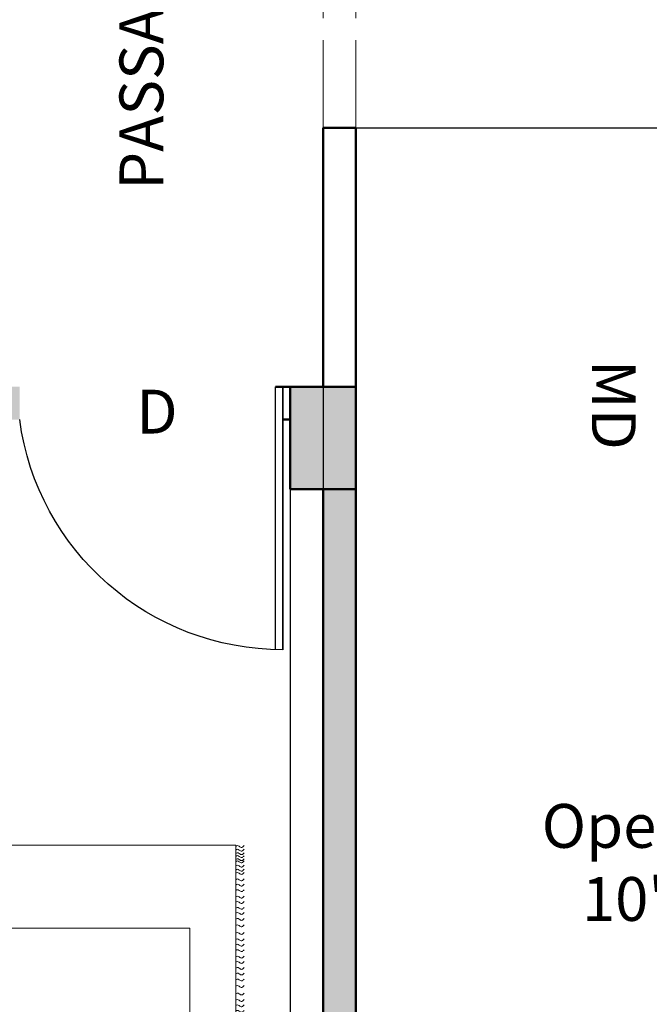
# Model space of a CAD drawing. Units: inches. Extents: x 1601 to 2080, y 5000 to 5589.
# Tile 4 of 11: x 1788 to 1874, y 5125 to 5259. Entities that reach past the tile are written whole.
import ezdxf

# ---------------------------------------------------------------- set-up
doc = ezdxf.new("R2010")
doc.units = ezdxf.units.IN
doc.header["$MEASUREMENT"] = 0
doc.linetypes.add('ACAD_ISO02W100', pattern=[15, 12, -3])
for name, color, linetype, lineweight in [('A-ANNO-DIMS', 2, 'Continuous', 18), ('A-ANNO-TEXT', 7, 'Continuous', 25), ('A-AREA-IDEN', 7, 'Continuous', 25), ('A-COLS', 7, 'Continuous', 50), ('A-COLS-PATT', 18, 'Continuous', 13), ('A-DOOR', 3, 'Continuous', 25), ('A-FLOR-PATT', 8, 'Continuous', 13), ('A-FURN', 8, 'Continuous', 18), ('A-WALL', 7, 'Continuous', 50), ('A-WALL-OVHD', 7, 'ACAD_ISO02W100', 18), ('A-WALL-PATT', 241, 'Continuous', 13)]:
    doc.layers.add(name, color=color, linetype=linetype, lineweight=lineweight)
doc.styles.get("Standard").update_dxf_attribs({"font": 'arial.ttf'})
doc.dimstyles.get("Standard").update_dxf_attribs({"dimtxt": 6, "dimasz": 0.18, "dimexe": 0.18, "dimexo": 0.0625, "dimgap": 0.09, "dimtad": 0, "dimtih": 1, "dimtoh": 1, "dimdec": 1, "dimzin": 0, "dimdsep": 46, "dimlunit": 3, "dimtxsty": 'Standard', "dimcen": 0.09, "dimadec": 0, "dimazin": 0, "dimtfac": 1, "dimtdec": 1, "dimtofl": 0, "dimtmove": 0, "dimatfit": 3, "dimfxl": 1, "dimtolj": 1, "dimtzin": 0, "dimarcsym": 0})

# ---------------------------------------------------------------- blocks, each defined once
blk = doc.blocks.new('BED-DOUBLE-ENSEMBLE')
for p, q in [((5.6, 61.61), (5.6, 51.56)), ((63.65, 61.72), (63.65, 51.66)), ((68.68, 56.69), (58.62, 56.69)), ((10.63, 56.59), (0.57, 56.59)), ((49.39, 52.82), (10.63, 52.82)), ((49.39, 52.82), (58, 46.47)), ((49.44, 52.82), (49.44, 46.47)), ((49.44, 52), (10.63, 52)), ((49.44, 46.47), (58, 46.47)), ((58.05, 34.96), (10.63, 34.96)), ((4.35, 0), (4.35, 26.37)), ((4.35, 26.37), (10.65, 26.37)), ((58.05, 26.37), (67.59, 26.37)), ((67.59, 26.37), (67.59, 0)), ((67.59, 0), (4.35, 0))]:
    blk.add_line(p, q)
for points in [[(0, 50.39), (10.63, 50.5), (10.63, 62.68), (0, 62.58)], [(58.05, 62.68), (58.05, 11.36), (10.63, 11.36), (10.63, 62.68)], [(58.05, 50.5), (68.68, 50.6), (68.68, 62.78), (58.05, 62.68)], [(29.88, 59.98), (29.88, 52.82), (15.98, 52.82), (15.98, 59.98)], [(49.44, 59.98), (49.44, 52.82), (35.55, 52.82), (35.55, 59.98)]]:
    blk.add_lwpolyline(points, close=True)
for centre in [(5.6, 56.59), (63.65, 56.69)]:
    blk.add_circle(centre, 3.92)
for points, knots in [([(3.23, 25.83), (3.32, 25.96), (3.52, 26.2), (3.86, 25.96), (4.14, 25.78), (4.29, 25.89), (4.35, 25.94)], [0, 0, 0, 0, 0.400747, 0.791423, 1.067667, 1.29709, 1.29709, 1.29709, 1.29709]), ([(68.71, 25.83), (68.61, 25.96), (68.42, 26.2), (68.08, 25.96), (67.8, 25.78), (67.65, 25.89), (67.58, 25.94)], [0, 0, 0, 0, 0.400747, 0.791423, 1.067667, 1.29709, 1.29709, 1.29709, 1.29709]), ([(3.23, 25.06), (3.32, 25.18), (3.52, 25.42), (3.86, 25.18), (4.14, 25), (4.29, 25.11), (4.35, 25.16)], [0, 0, 0, 0, 0.400747, 0.791423, 1.067667, 1.29709, 1.29709, 1.29709, 1.29709]), ([(3.23, 24.24), (3.32, 24.36), (3.52, 24.6), (3.86, 24.36), (4.14, 24.19), (4.29, 24.3), (4.35, 24.34)], [0, 0, 0, 0, 0.400747, 0.791423, 1.067667, 1.29709, 1.29709, 1.29709, 1.29709]), ([(68.71, 25.06), (68.61, 25.18), (68.42, 25.42), (68.08, 25.18), (67.8, 25), (67.65, 25.11), (67.58, 25.16)], [0, 0, 0, 0, 0.400747, 0.791423, 1.067667, 1.29709, 1.29709, 1.29709, 1.29709]), ([(68.71, 24.24), (68.61, 24.36), (68.42, 24.6), (68.08, 24.36), (67.8, 24.19), (67.65, 24.3), (67.58, 24.34)], [0, 0, 0, 0, 0.400747, 0.791423, 1.067667, 1.29709, 1.29709, 1.29709, 1.29709]), ([(3.23, 23.51), (3.32, 23.63), (3.52, 23.87), (3.86, 23.63), (4.14, 23.46), (4.29, 23.57), (4.35, 23.62)], [0, 0, 0, 0, 0.400747, 0.791423, 1.067667, 1.29709, 1.29709, 1.29709, 1.29709]), ([(68.71, 23.51), (68.61, 23.63), (68.42, 23.87), (68.08, 23.63), (67.8, 23.46), (67.65, 23.57), (67.58, 23.62)], [0, 0, 0, 0, 0.400747, 0.791423, 1.067667, 1.29709, 1.29709, 1.29709, 1.29709]), ([(3.23, 22.63), (3.32, 22.75), (3.52, 22.99), (3.86, 22.75), (4.14, 22.58), (4.29, 22.68), (4.35, 22.73)], [0, 0, 0, 0, 0.400747, 0.791423, 1.067667, 1.29709, 1.29709, 1.29709, 1.29709]), ([(3.23, 21.88), (3.32, 22), (3.52, 22.24), (3.86, 22), (4.14, 21.83), (4.29, 21.93), (4.35, 21.98)], [0, 0, 0, 0, 0.400747, 0.791423, 1.067667, 1.29709, 1.29709, 1.29709, 1.29709]), ([(68.71, 22.63), (68.61, 22.75), (68.42, 22.99), (68.08, 22.75), (67.8, 22.58), (67.65, 22.68), (67.58, 22.73)], [0, 0, 0, 0, 0.400747, 0.791423, 1.067667, 1.29709, 1.29709, 1.29709, 1.29709]), ([(68.71, 21.88), (68.61, 22), (68.42, 22.24), (68.08, 22), (67.8, 21.83), (67.65, 21.93), (67.58, 21.98)], [0, 0, 0, 0, 0.400747, 0.791423, 1.067667, 1.29709, 1.29709, 1.29709, 1.29709]), ([(3.23, 21.15), (3.32, 21.27), (3.52, 21.51), (3.86, 21.27), (4.14, 21.1), (4.29, 21.2), (4.35, 21.25)], [0, 0, 0, 0, 0.400747, 0.791423, 1.067667, 1.29709, 1.29709, 1.29709, 1.29709]), ([(3.23, 20.27), (3.32, 20.39), (3.52, 20.63), (3.86, 20.39), (4.14, 20.22), (4.29, 20.32), (4.35, 20.37)], [0, 0, 0, 0, 0.400747, 0.791423, 1.067667, 1.29709, 1.29709, 1.29709, 1.29709]), ([(68.71, 21.15), (68.61, 21.27), (68.42, 21.51), (68.08, 21.27), (67.8, 21.1), (67.65, 21.2), (67.58, 21.25)], [0, 0, 0, 0, 0.400747, 0.791423, 1.067667, 1.29709, 1.29709, 1.29709, 1.29709]), ([(68.71, 20.27), (68.61, 20.39), (68.42, 20.63), (68.08, 20.39), (67.8, 20.22), (67.65, 20.32), (67.58, 20.37)], [0, 0, 0, 0, 0.400747, 0.791423, 1.067667, 1.29709, 1.29709, 1.29709, 1.29709]), ([(3.23, 19.23), (3.32, 19.35), (3.52, 19.59), (3.86, 19.35), (4.14, 19.18), (4.29, 19.29), (4.35, 19.33)], [0, 0, 0, 0, 0.400747, 0.791423, 1.067667, 1.29709, 1.29709, 1.29709, 1.29709]), ([(68.71, 19.23), (68.61, 19.35), (68.42, 19.59), (68.08, 19.35), (67.8, 19.18), (67.65, 19.29), (67.58, 19.33)], [0, 0, 0, 0, 0.400747, 0.791423, 1.067667, 1.29709, 1.29709, 1.29709, 1.29709]), ([(3.23, 18.35), (3.32, 18.47), (3.52, 18.71), (3.86, 18.47), (4.14, 18.3), (4.29, 18.4), (4.35, 18.45)], [0, 0, 0, 0, 0.400747, 0.791423, 1.067667, 1.29709, 1.29709, 1.29709, 1.29709]), ([(3.23, 17.53), (3.32, 17.65), (3.52, 17.89), (3.86, 17.65), (4.14, 17.48), (4.29, 17.59), (4.35, 17.64)], [0, 0, 0, 0, 0.400747, 0.791423, 1.067667, 1.29709, 1.29709, 1.29709, 1.29709]), ([(68.71, 18.35), (68.61, 18.47), (68.42, 18.71), (68.08, 18.47), (67.8, 18.3), (67.65, 18.4), (67.58, 18.45)], [0, 0, 0, 0, 0.400747, 0.791423, 1.067667, 1.29709, 1.29709, 1.29709, 1.29709]), ([(68.71, 17.53), (68.61, 17.65), (68.42, 17.89), (68.08, 17.65), (67.8, 17.48), (67.65, 17.59), (67.58, 17.64)], [0, 0, 0, 0, 0.400747, 0.791423, 1.067667, 1.29709, 1.29709, 1.29709, 1.29709]), ([(3.23, 16.76), (3.32, 16.88), (3.52, 17.12), (3.86, 16.88), (4.14, 16.7), (4.29, 16.81), (4.35, 16.86)], [0, 0, 0, 0, 0.400747, 0.791423, 1.067667, 1.29709, 1.29709, 1.29709, 1.29709]), ([(3.23, 15.94), (3.32, 16.06), (3.52, 16.3), (3.86, 16.06), (4.14, 15.89), (4.29, 15.99), (4.35, 16.04)], [0, 0, 0, 0, 0.400747, 0.791423, 1.067667, 1.29709, 1.29709, 1.29709, 1.29709]), ([(68.71, 16.76), (68.61, 16.88), (68.42, 17.12), (68.08, 16.88), (67.8, 16.7), (67.65, 16.81), (67.58, 16.86)], [0, 0, 0, 0, 0.400747, 0.791423, 1.067667, 1.29709, 1.29709, 1.29709, 1.29709]), ([(68.71, 15.94), (68.61, 16.06), (68.42, 16.3), (68.08, 16.06), (67.8, 15.89), (67.65, 15.99), (67.58, 16.04)], [0, 0, 0, 0, 0.400747, 0.791423, 1.067667, 1.29709, 1.29709, 1.29709, 1.29709]), ([(3.23, 15.21), (3.32, 15.33), (3.52, 15.57), (3.86, 15.33), (4.14, 15.16), (4.29, 15.27), (4.35, 15.31)], [0, 0, 0, 0, 0.400747, 0.791423, 1.067667, 1.29709, 1.29709, 1.29709, 1.29709]), ([(68.71, 15.21), (68.61, 15.33), (68.42, 15.57), (68.08, 15.33), (67.8, 15.16), (67.65, 15.27), (67.58, 15.31)], [0, 0, 0, 0, 0.400747, 0.791423, 1.067667, 1.29709, 1.29709, 1.29709, 1.29709]), ([(3.23, 14.33), (3.32, 14.45), (3.52, 14.69), (3.86, 14.45), (4.14, 14.28), (4.29, 14.38), (4.35, 14.43)], [0, 0, 0, 0, 0.400747, 0.791423, 1.067667, 1.29709, 1.29709, 1.29709, 1.29709]), ([(3.23, 13.58), (3.32, 13.7), (3.52, 13.94), (3.86, 13.7), (4.14, 13.53), (4.29, 13.63), (4.35, 13.68)], [0, 0, 0, 0, 0.400747, 0.791423, 1.067667, 1.29709, 1.29709, 1.29709, 1.29709]), ([(68.71, 14.33), (68.61, 14.45), (68.42, 14.69), (68.08, 14.45), (67.8, 14.28), (67.65, 14.38), (67.58, 14.43)], [0, 0, 0, 0, 0.400747, 0.791423, 1.067667, 1.29709, 1.29709, 1.29709, 1.29709]), ([(68.71, 13.58), (68.61, 13.7), (68.42, 13.94), (68.08, 13.7), (67.8, 13.53), (67.65, 13.63), (67.58, 13.68)], [0, 0, 0, 0, 0.400747, 0.791423, 1.067667, 1.29709, 1.29709, 1.29709, 1.29709]), ([(3.23, 12.85), (3.32, 12.97), (3.52, 13.21), (3.86, 12.97), (4.14, 12.8), (4.29, 12.9), (4.35, 12.95)], [0, 0, 0, 0, 0.400747, 0.791423, 1.067667, 1.29709, 1.29709, 1.29709, 1.29709]), ([(3.23, 11.97), (3.32, 12.09), (3.52, 12.33), (3.86, 12.09), (4.14, 11.92), (4.29, 12.02), (4.35, 12.07)], [0, 0, 0, 0, 0.400747, 0.791423, 1.067667, 1.29709, 1.29709, 1.29709, 1.29709]), ([(68.71, 12.85), (68.61, 12.97), (68.42, 13.21), (68.08, 12.97), (67.8, 12.8), (67.65, 12.9), (67.58, 12.95)], [0, 0, 0, 0, 0.400747, 0.791423, 1.067667, 1.29709, 1.29709, 1.29709, 1.29709]), ([(68.71, 11.97), (68.61, 12.09), (68.42, 12.33), (68.08, 12.09), (67.8, 11.92), (67.65, 12.02), (67.58, 12.07)], [0, 0, 0, 0, 0.400747, 0.791423, 1.067667, 1.29709, 1.29709, 1.29709, 1.29709]), ([(3.23, 10.93), (3.32, 11.05), (3.52, 11.29), (3.86, 11.05), (4.14, 10.88), (4.29, 10.99), (4.35, 11.03)], [0, 0, 0, 0, 0.400747, 0.791423, 1.067667, 1.29709, 1.29709, 1.29709, 1.29709]), ([(68.71, 10.93), (68.61, 11.05), (68.42, 11.29), (68.08, 11.05), (67.8, 10.88), (67.65, 10.99), (67.58, 11.03)], [0, 0, 0, 0, 0.400747, 0.791423, 1.067667, 1.29709, 1.29709, 1.29709, 1.29709]), ([(3.23, 10.05), (3.32, 10.17), (3.52, 10.41), (3.86, 10.17), (4.14, 10), (4.29, 10.1), (4.35, 10.15)], [0, 0, 0, 0, 0.400747, 0.791423, 1.067667, 1.29709, 1.29709, 1.29709, 1.29709]), ([(3.23, 9.23), (3.32, 9.35), (3.52, 9.59), (3.86, 9.35), (4.14, 9.18), (4.29, 9.29), (4.35, 9.34)], [0, 0, 0, 0, 0.400747, 0.791423, 1.067667, 1.29709, 1.29709, 1.29709, 1.29709]), ([(68.71, 10.05), (68.61, 10.17), (68.42, 10.41), (68.08, 10.17), (67.8, 10), (67.65, 10.1), (67.58, 10.15)], [0, 0, 0, 0, 0.400747, 0.791423, 1.067667, 1.29709, 1.29709, 1.29709, 1.29709]), ([(68.71, 9.23), (68.61, 9.35), (68.42, 9.59), (68.08, 9.35), (67.8, 9.18), (67.65, 9.29), (67.58, 9.34)], [0, 0, 0, 0, 0.400747, 0.791423, 1.067667, 1.29709, 1.29709, 1.29709, 1.29709]), ([(3.23, 8.54), (3.32, 8.66), (3.52, 8.9), (3.86, 8.66), (4.14, 8.49), (4.29, 8.6), (4.35, 8.65)], [0, 0, 0, 0, 0.400747, 0.791423, 1.067667, 1.29709, 1.29709, 1.29709, 1.29709]), ([(68.71, 8.54), (68.61, 8.66), (68.42, 8.9), (68.08, 8.66), (67.8, 8.49), (67.65, 8.6), (67.58, 8.65)], [0, 0, 0, 0, 0.400747, 0.791423, 1.067667, 1.29709, 1.29709, 1.29709, 1.29709]), ([(3.23, 7.73), (3.32, 7.85), (3.52, 8.09), (3.86, 7.85), (4.14, 7.67), (4.29, 7.78), (4.35, 7.83)], [0, 0, 0, 0, 0.400747, 0.791423, 1.067667, 1.29709, 1.29709, 1.29709, 1.29709]), ([(3.23, 7), (3.32, 7.12), (3.52, 7.36), (3.86, 7.12), (4.14, 6.95), (4.29, 7.05), (4.35, 7.1)], [0, 0, 0, 0, 0.400747, 0.791423, 1.067667, 1.29709, 1.29709, 1.29709, 1.29709]), ([(68.71, 7.73), (68.61, 7.85), (68.42, 8.09), (68.08, 7.85), (67.8, 7.67), (67.65, 7.78), (67.58, 7.83)], [0, 0, 0, 0, 0.400747, 0.791423, 1.067667, 1.29709, 1.29709, 1.29709, 1.29709]), ([(68.71, 7), (68.61, 7.12), (68.42, 7.36), (68.08, 7.12), (67.8, 6.95), (67.65, 7.05), (67.58, 7.1)], [0, 0, 0, 0, 0.400747, 0.791423, 1.067667, 1.29709, 1.29709, 1.29709, 1.29709]), ([(3.23, 6.12), (3.32, 6.24), (3.52, 6.48), (3.86, 6.24), (4.14, 6.06), (4.29, 6.17), (4.35, 6.22)], [0, 0, 0, 0, 0.400747, 0.791423, 1.067667, 1.29709, 1.29709, 1.29709, 1.29709]), ([(3.23, 5.36), (3.32, 5.49), (3.52, 5.72), (3.86, 5.49), (4.14, 5.31), (4.29, 5.42), (4.35, 5.47)], [0, 0, 0, 0, 0.400747, 0.791423, 1.067667, 1.29709, 1.29709, 1.29709, 1.29709]), ([(68.71, 6.12), (68.61, 6.24), (68.42, 6.48), (68.08, 6.24), (67.8, 6.06), (67.65, 6.17), (67.58, 6.22)], [0, 0, 0, 0, 0.400747, 0.791423, 1.067667, 1.29709, 1.29709, 1.29709, 1.29709]), ([(68.71, 5.36), (68.61, 5.49), (68.42, 5.72), (68.08, 5.49), (67.8, 5.31), (67.65, 5.42), (67.58, 5.47)], [0, 0, 0, 0, 0.400747, 0.791423, 1.067667, 1.29709, 1.29709, 1.29709, 1.29709]), ([(3.23, 4.64), (3.32, 4.76), (3.52, 5), (3.86, 4.76), (4.14, 4.58), (4.29, 4.69), (4.35, 4.74)], [0, 0, 0, 0, 0.400747, 0.791423, 1.067667, 1.29709, 1.29709, 1.29709, 1.29709]), ([(68.71, 4.64), (68.61, 4.76), (68.42, 5), (68.08, 4.76), (67.8, 4.59), (67.66, 4.69), (67.59, 4.73)], [0, 0, 0, 0, 0.400747, 0.791423, 1.067667, 1.283686, 1.283686, 1.283686, 1.283686]), ([(3.23, 3.75), (3.32, 3.88), (3.52, 4.11), (3.86, 3.88), (4.14, 3.7), (4.29, 3.81), (4.35, 3.86)], [0, 0, 0, 0, 0.400747, 0.791423, 1.067667, 1.29709, 1.29709, 1.29709, 1.29709]), ([(3.23, 3.32), (3.32, 3.45), (3.51, 3.7), (3.86, 3.44), (4.14, 3.27), (4.29, 3.38), (4.35, 3.43)], [0, 0, 0, 0, 0.407265, 0.802015, 1.07826, 1.307683, 1.307683, 1.307683, 1.307683]), ([(3.23, 2.76), (3.32, 2.88), (3.52, 3.12), (3.86, 2.88), (4.14, 2.71), (4.29, 2.81), (4.35, 2.86)], [0, 0, 0, 0, 0.400747, 0.791423, 1.067667, 1.29709, 1.29709, 1.29709, 1.29709]), ([(68.71, 3.75), (68.61, 3.88), (68.42, 4.11), (68.08, 3.88), (67.8, 3.7), (67.66, 3.8), (67.59, 3.85)], [0, 0, 0, 0, 0.400747, 0.791423, 1.067667, 1.283686, 1.283686, 1.283686, 1.283686]), ([(68.71, 3.32), (68.61, 3.45), (68.42, 3.69), (68.08, 3.45), (67.8, 3.27), (67.66, 3.38), (67.59, 3.42)], [0, 0, 0, 0, 0.402903, 0.794912, 1.071156, 1.287177, 1.287177, 1.287177, 1.287177]), ([(68.71, 2.73), (68.61, 2.85), (68.42, 3.09), (68.08, 2.85), (67.8, 2.68), (67.66, 2.78), (67.59, 2.82)], [0, 0, 0, 0, 0.400747, 0.791423, 1.067667, 1.283686, 1.283686, 1.283686, 1.283686]), ([(3.23, 2.18), (3.32, 2.31), (3.52, 2.54), (3.86, 2.31), (4.14, 2.13), (4.29, 2.24), (4.35, 2.29)], [0, 0, 0, 0, 0.400747, 0.791423, 1.067667, 1.29709, 1.29709, 1.29709, 1.29709]), ([(3.23, 1.88), (3.32, 2), (3.52, 2.24), (3.86, 2), (4.14, 1.82), (4.29, 1.93), (4.35, 1.98)], [0, 0, 0, 0, 0.400747, 0.791423, 1.067667, 1.29709, 1.29709, 1.29709, 1.29709]), ([(3.23, 1.46), (3.32, 1.58), (3.52, 1.82), (3.86, 1.58), (4.14, 1.4), (4.29, 1.51), (4.35, 1.56)], [0, 0, 0, 0, 0.400747, 0.791423, 1.067667, 1.29709, 1.29709, 1.29709, 1.29709]), ([(68.71, 1.43), (68.61, 1.55), (68.42, 1.79), (68.08, 1.55), (67.8, 1.38), (67.65, 1.48), (67.58, 1.53)], [0, 0, 0, 0, 0.400747, 0.791423, 1.067667, 1.29709, 1.29709, 1.29709, 1.29709]), ([(68.71, 2.16), (68.61, 2.28), (68.42, 2.52), (68.08, 2.28), (67.8, 2.11), (67.66, 2.21), (67.59, 2.25)], [0, 0, 0, 0, 0.400747, 0.791423, 1.067667, 1.283686, 1.283686, 1.283686, 1.283686]), ([(68.71, 1.85), (68.61, 1.97), (68.42, 2.21), (68.08, 1.97), (67.8, 1.8), (67.66, 1.9), (67.59, 1.94)], [0, 0, 0, 0, 0.400747, 0.791423, 1.067667, 1.283686, 1.283686, 1.283686, 1.283686]), ([(3.23, 1.06), (3.32, 1.18), (3.52, 1.42), (3.86, 1.18), (4.14, 1.01), (4.29, 1.11), (4.35, 1.16)], [0, 0, 0, 0, 0.400747, 0.791423, 1.067667, 1.29709, 1.29709, 1.29709, 1.29709]), ([(3.23, 0.57), (3.32, 0.7), (3.52, 0.93), (3.86, 0.7), (4.14, 0.52), (4.29, 0.63), (4.35, 0.68)], [0, 0, 0, 0, 0.400747, 0.791423, 1.067667, 1.29709, 1.29709, 1.29709, 1.29709]), ([(3.23, 0.07), (3.32, 0.19), (3.52, 0.43), (3.86, 0.19), (4.14, 0.02), (4.29, 0.13), (4.35, 0.18)], [0, 0, 0, 0, 0.400747, 0.791423, 1.067667, 1.29709, 1.29709, 1.29709, 1.29709]), ([(68.71, 1.03), (68.61, 1.15), (68.42, 1.39), (68.08, 1.15), (67.8, 0.98), (67.65, 1.09), (67.58, 1.13)], [0, 0, 0, 0, 0.400747, 0.791423, 1.067667, 1.29709, 1.29709, 1.29709, 1.29709]), ([(68.71, 0.55), (68.61, 0.67), (68.42, 0.91), (68.08, 0.67), (67.8, 0.49), (67.65, 0.6), (67.58, 0.65)], [0, 0, 0, 0, 0.400747, 0.791423, 1.067667, 1.29709, 1.29709, 1.29709, 1.29709]), ([(68.71, 0.07), (68.61, 0.19), (68.42, 0.43), (68.08, 0.19), (67.8, 0.02), (67.65, 0.13), (67.58, 0.18)], [0, 0, 0, 0, 0.400747, 0.791423, 1.067667, 1.29709, 1.29709, 1.29709, 1.29709])]:
    blk.add_open_spline(points, degree=3, knots=knots)
blk = doc.blocks.new('DOOR-36IN')
for p, q in [((35, 36), (35, 0)), ((36, 0), (36, 36)), ((36, 36), (36, 0)), ((36, 0), (35, 0))]:
    blk.add_line(p, q)
blk.add_arc((36, -0.32), 36.32, 90, 172.3719)
blk = doc.blocks.new('*D56')
at = {"layer": 'A-ANNO-DIMS', "color": 0, "lineweight": -2, "transparency": 16777216}
for p, q in [((1833.97, 5300.2), (2047.44, 5300.2)), ((2047.26, 5300.02), (2047.26, 5275.61)), ((2047.26, 5244.82), (2047.26, 5269.23)), ((1833.97, 5244.64), (2047.44, 5244.64))]:
    blk.add_line(p, q, dxfattribs=at)
at = {"layer": 'A-ANNO-DIMS', "color": 0, "transparency": 16777216}
for points in [[(2047.23, 5300.02), (2047.29, 5300.02), (2047.26, 5300.2)], [(2047.23, 5244.82), (2047.29, 5244.82), (2047.26, 5244.64)]]:
    blk.add_solid(points, dxfattribs=at)
at = {"layer": 'Defpoints', "color": 0, "transparency": 16777216}
for p in [(1833.91, 5300.2), (2047.26, 5300.2), (1833.91, 5244.64)]:
    blk.add_point(p, dxfattribs=at)
at = {"layer": 'A-ANNO-DIMS', "color": 0, "transparency": 16777216, "insert": (2047.26, 5272.42), "char_height": 6, "attachment_point": 5}
blk.add_mtext('\\A1;4\'-7 1/2"', dxfattribs=at)
blk = doc.blocks.new('*D57')
at = {"layer": 'A-ANNO-DIMS', "color": 0, "lineweight": -2, "transparency": 16777216}
for p, q in [((1829.41, 5244.58), (1829.41, 5022.68)), ((1833.91, 5244.58), (1833.91, 5022.68)), ((1829.59, 5022.86), (1833.73, 5022.86)), ((1833.91, 5022.86), (1834.09, 5022.86))]:
    blk.add_line(p, q, dxfattribs=at)
at = {"layer": 'A-ANNO-DIMS', "color": 0, "transparency": 16777216}
for points in [[(1829.59, 5022.89), (1829.59, 5022.83), (1829.41, 5022.86)], [(1833.73, 5022.89), (1833.73, 5022.83), (1833.91, 5022.86)]]:
    blk.add_solid(points, dxfattribs=at)
at = {"layer": 'Defpoints', "color": 0, "transparency": 16777216}
for p in [(1829.41, 5244.64), (1833.91, 5244.64), (1833.91, 5022.86)]:
    blk.add_point(p, dxfattribs=at)
at = {"layer": 'A-ANNO-DIMS', "color": 0, "transparency": 16777216, "insert": (1849.14, 5022.86), "char_height": 6, "attachment_point": 5}
blk.add_mtext('\\A1;0\'-4 1/2"', dxfattribs=at)
blk = doc.blocks.new('*D58')
at = {"layer": 'A-ANNO-DIMS', "color": 0, "lineweight": -2, "transparency": 16777216}
for p, q in [((1779.91, 5209.13), (1779.91, 5022.68)), ((1824.91, 5209.13), (1824.91, 5022.68)), ((1780.09, 5022.86), (1794.35, 5022.86)), ((1824.73, 5022.86), (1810.47, 5022.86))]:
    blk.add_line(p, q, dxfattribs=at)
at = {"layer": 'A-ANNO-DIMS', "color": 0, "transparency": 16777216}
for points in [[(1780.09, 5022.89), (1780.09, 5022.83), (1779.91, 5022.86)], [(1824.73, 5022.89), (1824.73, 5022.83), (1824.91, 5022.86)]]:
    blk.add_solid(points, dxfattribs=at)
at = {"layer": 'Defpoints', "color": 0, "transparency": 16777216}
for p in [(1779.91, 5209.2), (1824.91, 5209.2), (1824.91, 5022.86)]:
    blk.add_point(p, dxfattribs=at)
at = {"layer": 'A-ANNO-DIMS', "color": 0, "transparency": 16777216, "insert": (1802.41, 5022.86), "char_height": 6, "attachment_point": 5}
blk.add_mtext('\\A1;3\'-9"', dxfattribs=at)

msp = doc.modelspace()

# ---------------------------------------------------------------- hatches: boundary and pattern name
at = {"layer": 'A-COLS-PATT'}
h = msp.add_hatch(color=256, dxfattribs=at)
h.dxf.hatch_style = 1
h.paths.add_polyline_path([(1702.41, 5431.2), (1688.41, 5431.2), (1688.41, 5422.2), (1702.41, 5422.2)])
h.paths.add_polyline_path([(1836.17, 5431.2), (1822.17, 5431.2), (1822.17, 5422.2), (1836.17, 5422.2)])
h.paths.add_polyline_path([(1962.91, 5431.2), (1948.91, 5431.2), (1948.91, 5422.2), (1962.91, 5422.2)])
h.paths.add_polyline_path([(1697.41, 5314.2), (1688.41, 5314.2), (1688.41, 5300.2), (1697.41, 5300.2)])
h.paths.add_polyline_path([(1833.91, 5314.2), (1824.91, 5314.2), (1824.91, 5300.2), (1833.91, 5300.2)])
h.paths.add_polyline_path([(1962.91, 5314.2), (1953.91, 5314.2), (1953.91, 5300.2), (1962.91, 5300.2)])
h.paths.add_polyline_path([(1697.41, 5209.2), (1688.41, 5209.2), (1688.41, 5195.2), (1697.41, 5195.2)])
h.paths.add_polyline_path([(1833.91, 5209.2), (1824.91, 5209.2), (1824.91, 5195.2), (1833.91, 5195.2)])
h.paths.add_polyline_path([(1962.91, 5209.2), (1953.91, 5209.2), (1953.91, 5195.2), (1962.91, 5195.2)])
h.paths.add_polyline_path([(1697.41, 5083.7), (1688.41, 5083.7), (1688.41, 5069.7), (1697.41, 5069.7)])
h.paths.add_polyline_path([(1833.91, 5078.7), (1819.91, 5078.7), (1819.91, 5069.7), (1833.91, 5069.7)])
h.paths.add_polyline_path([(1962.91, 5078.7), (1948.91, 5078.7), (1948.91, 5069.7), (1962.91, 5069.7)])
at = {"layer": 'A-FLOR-PATT'}
h = msp.add_hatch(dxfattribs=at)
h.set_pattern_fill('ANGLE', color=256, scale=40)
h.set_pattern_definition([(0, (0, 0), (0, 11), [8, -3]), (90, (0, 0), (-11, 7e-16), [8, -3])])
h.paths.add_polyline_path([(2022.91, 5509.2), (1941.91, 5509.2), (1911.91, 5509.2), (1864.41, 5509.2), (1864.41, 5489.7), (1868.54, 5489.7, -0.022155), (1868.52, 5490.01, -1), (1875.53, 5490.01, -0.956651), (1868.54, 5489.7), (1864.41, 5489.7), (1864.41, 5470.2), (1794.41, 5470.2), (1794.41, 5431.2), (1811.95, 5431.2), (1911.91, 5431.2), (1941.91, 5431.2), (1942.91, 5431.2), (1945.91, 5431.2), (1948.91, 5431.2), (1962.91, 5431.2), (1962.91, 5415.29), (1962.91, 5385.29), (1962.91, 5384.29), (1962.91, 5381.29), (1962.91, 5333.29), (1962.91, 5069.7), (2022.91, 5069.7)])
h.paths.add_polyline_path([(2000.28, 5267.55), (2000.28, 5367.64), (1987.91, 5367.64), (1987.91, 5267.55)], flags=24)
h.paths.add_polyline_path([(1879.42, 5455.52), (1969.04, 5455.52), (1969.04, 5467.88), (1879.42, 5467.88)], flags=24)
at = {"layer": 'A-WALL-PATT'}
h = msp.add_hatch(color=256, dxfattribs=at)
h.dxf.hatch_style = 1
h.paths.add_polyline_path([(1763.95, 5431.2), (1702.41, 5431.2), (1702.41, 5422.2), (1763.95, 5422.2)])
h.paths.add_polyline_path([(1697.41, 5422.2), (1688.41, 5422.2), (1688.41, 5314.2), (1697.41, 5314.2)])
h.paths.add_polyline_path([(1740.41, 5314.2), (1697.41, 5314.2), (1697.41, 5309.7), (1740.41, 5309.7)], flags=17)
h.paths.add_polyline_path([(1822.17, 5431.2), (1811.95, 5431.2), (1811.95, 5422.2), (1822.17, 5422.2)])
h.paths.add_polyline_path([(1845.52, 5431.2), (1836.17, 5431.2), (1836.17, 5422.2), (1845.52, 5422.2)])
h.paths.add_polyline_path([(1910.91, 5431.2), (1881.52, 5431.2), (1881.52, 5422.2), (1910.91, 5422.2)])
h.paths.add_polyline_path([(1948.91, 5431.2), (1945.91, 5431.2), (1942.91, 5431.2), (1942.91, 5422.2), (1948.91, 5422.2)])
h.paths.add_polyline_path([(1962.91, 5422.2), (1953.91, 5422.2), (1953.91, 5416.29), (1962.91, 5416.29)])
h.paths.add_polyline_path([(1962.91, 5384.29), (1953.91, 5384.29), (1953.91, 5381.29), (1962.91, 5381.29)])
h.paths.add_polyline_path([(1962.91, 5333.29), (1953.91, 5333.29), (1953.91, 5314.2), (1962.91, 5314.2)])
h.paths.add_polyline_path([(1962.91, 5300.2), (1953.91, 5300.2), (1953.91, 5236.2), (1875.91, 5236.2), (1875.91, 5230.7), (1881.91, 5230.7), (1881.91, 5231.7), (1953.91, 5231.7), (1953.91, 5219.2), (1962.91, 5219.2)])
h.paths.add_polyline_path([(1962.91, 5185.2), (1953.91, 5185.2), (1953.91, 5183.7), (1881.91, 5183.7), (1881.91, 5184.7), (1875.91, 5184.7), (1875.91, 5183.7), (1875.91, 5179.2), (1953.91, 5179.2), (1953.91, 5172.6), (1962.91, 5172.6)])
h.paths.add_polyline_path([(1962.91, 5136.6), (1953.91, 5136.6), (1953.91, 5078.7), (1962.91, 5078.7)])
h.paths.add_polyline_path([(1948.91, 5078.7), (1833.91, 5078.7), (1833.91, 5069.7), (1948.91, 5069.7)])
h.paths.add_polyline_path([(1833.91, 5195.2), (1829.41, 5195.2), (1829.41, 5078.7), (1833.91, 5078.7)])
h.paths.add_polyline_path([(1819.91, 5078.7), (1813.58, 5078.7), (1813.58, 5069.7), (1819.91, 5069.7)])
h.paths.add_polyline_path([(1765.58, 5078.7), (1697.41, 5078.7), (1697.41, 5069.7), (1765.58, 5069.7)])
h.paths.add_polyline_path([(1697.41, 5195.2), (1688.41, 5195.2), (1688.41, 5083.7), (1697.41, 5083.7)])
h.paths.add_polyline_path([(1740.41, 5209.2), (1697.41, 5209.2), (1697.41, 5204.7), (1740.41, 5204.7)], flags=17)
h.paths.add_polyline_path([(1787.91, 5209.2), (1779.91, 5209.2), (1779.91, 5309.7), (1787.91, 5309.7), (1787.91, 5314.2), (1772.41, 5314.2), (1772.41, 5309.7), (1775.41, 5309.7), (1775.41, 5261.7), (1697.41, 5261.7), (1697.41, 5273.07), (1688.41, 5273.07), (1688.41, 5242.37), (1697.41, 5242.37), (1697.41, 5257.2), (1775.41, 5257.2), (1775.41, 5209.2), (1772.41, 5209.2), (1772.41, 5204.7), (1775.41, 5204.7), (1787.91, 5204.7)])
h.paths.add_polyline_path([(1697.41, 5218.37), (1688.41, 5218.37), (1688.41, 5209.2), (1697.41, 5209.2)], flags=17)
h.paths.add_polyline_path([(1833.91, 5422.2), (1829.41, 5422.2), (1829.41, 5314.2), (1833.91, 5314.2)])
h.paths.add_polyline_path([(1697.41, 5300.2), (1688.41, 5300.2), (1688.41, 5297.07), (1697.41, 5297.07)], flags=17)

# ---------------------------------------------------------------- linework, layer by layer
at = {"layer": 'A-COLS'}
for p, q in [((1833.91, 5209.2), (1824.91, 5209.2)), ((1824.91, 5209.2), (1824.91, 5195.2)), ((1824.91, 5195.2), (1833.91, 5195.2))]:
    msp.add_line(p, q, dxfattribs=at)
at = {"layer": 'A-WALL'}
for p, q in [((1829.41, 5244.64), (1829.41, 5209.2)), ((1829.41, 5244.64), (1833.91, 5244.64)), ((1833.91, 5244.64), (1833.91, 5069.7)), ((1822.91, 5209.2), (1833.91, 5209.2)), ((1824.91, 5209.2), (1823.91, 5209.2)), ((1823.91, 5204.7), (1824.91, 5204.7)), ((1829.41, 5195.2), (1829.41, 5078.7))]:
    msp.add_line(p, q, dxfattribs=at)
at = {"layer": 'A-WALL-OVHD'}
for p, q in [((1829.41, 5244.64), (1829.41, 5300.2)), ((1833.91, 5244.64), (1833.91, 5300.2))]:
    msp.add_line(p, q, dxfattribs=at)

# ---------------------------------------------------------------- block references
at = {"layer": 'A-DOOR', "extrusion": (0, 0, -1), "zscale": -1, "rotation": 180}
msp.add_blockref('DOOR-36IN', (-1787.91, 5209.2), dxfattribs=at)
at = {"layer": 'A-FURN', "rotation": 180}
msp.add_blockref('BED-DOUBLE-ENSEMBLE', (1821.83, 5146.47), dxfattribs=at)

# ---------------------------------------------------------------- texts
at = {"layer": 'A-ANNO-TEXT', "insert": (1872.19, 5212.85), "char_height": 6, "attachment_point": 1, "rotation": 270}
msp.add_mtext_dynamic_manual_height_columns('MD', width=13.3594, gutter_width=30, heights=[0], dxfattribs=at)
at = {"layer": 'A-ANNO-TEXT', "insert": (1803.88, 5208.8), "char_height": 6, "attachment_point": 1}
msp.add_mtext_dynamic_manual_height_columns('D ', width=9.7695, gutter_width=30, heights=[0], dxfattribs=at)
at = {"layer": 'A-AREA-IDEN', "insert": (1801.56, 5236.17), "char_height": 6, "attachment_point": 1, "rotation": 90}
msp.add_mtext_dynamic_manual_height_columns('PASSAGE', width=39.5906, gutter_width=30, heights=[0], dxfattribs=at)
at = {"layer": 'A-AREA-IDEN', "insert": (1859.33, 5152.09), "char_height": 6, "attachment_point": 1}
msp.add_mtext_dynamic_manual_height_columns('Open kitchen\\P   10\'0"x8\'6"', width=60.0959, gutter_width=30, heights=[0], dxfattribs=at)

# ---------------------------------------------------------------- dimensions: what is measured, and where the dimension line sits
at = {"layer": 'A-ANNO-DIMS'}
dim = msp.add_linear_dim(base=(2047.26, 5300.2), p1=(1833.91, 5244.64), p2=(1833.91, 5300.2), angle=90, dimstyle='Standard', override={"dimdec": 1, "dimlfac": 1, "dimrnd": 0, "dimzin": 1, "dimdsep": 46, "dimlunit": 4, "dimfrac": 2}, dxfattribs=at)
dim.commit()
dim.dimension.update_dxf_attribs({"geometry": '*D56', "text_midpoint": (2047.26, 5272.42)})
for base, p1, p2, picture, middle in [((1833.91, 5022.86), (1829.41, 5244.64), (1833.91, 5244.64), '*D57', (1849.14, 5022.86)), ((1824.91, 5022.86), (1779.91, 5209.2), (1824.91, 5209.2), '*D58', (1802.41, 5022.86))]:
    dim = msp.add_linear_dim(base=base, p1=p1, p2=p2, dimstyle='Standard', override={"dimdec": 1, "dimlfac": 1, "dimrnd": 0, "dimzin": 1, "dimdsep": 46, "dimlunit": 4, "dimfrac": 2}, dxfattribs=at)
    dim.commit()
    dim.dimension.update_dxf_attribs({"geometry": picture, "text_midpoint": middle})

doc.saveas('drawing.dxf')
